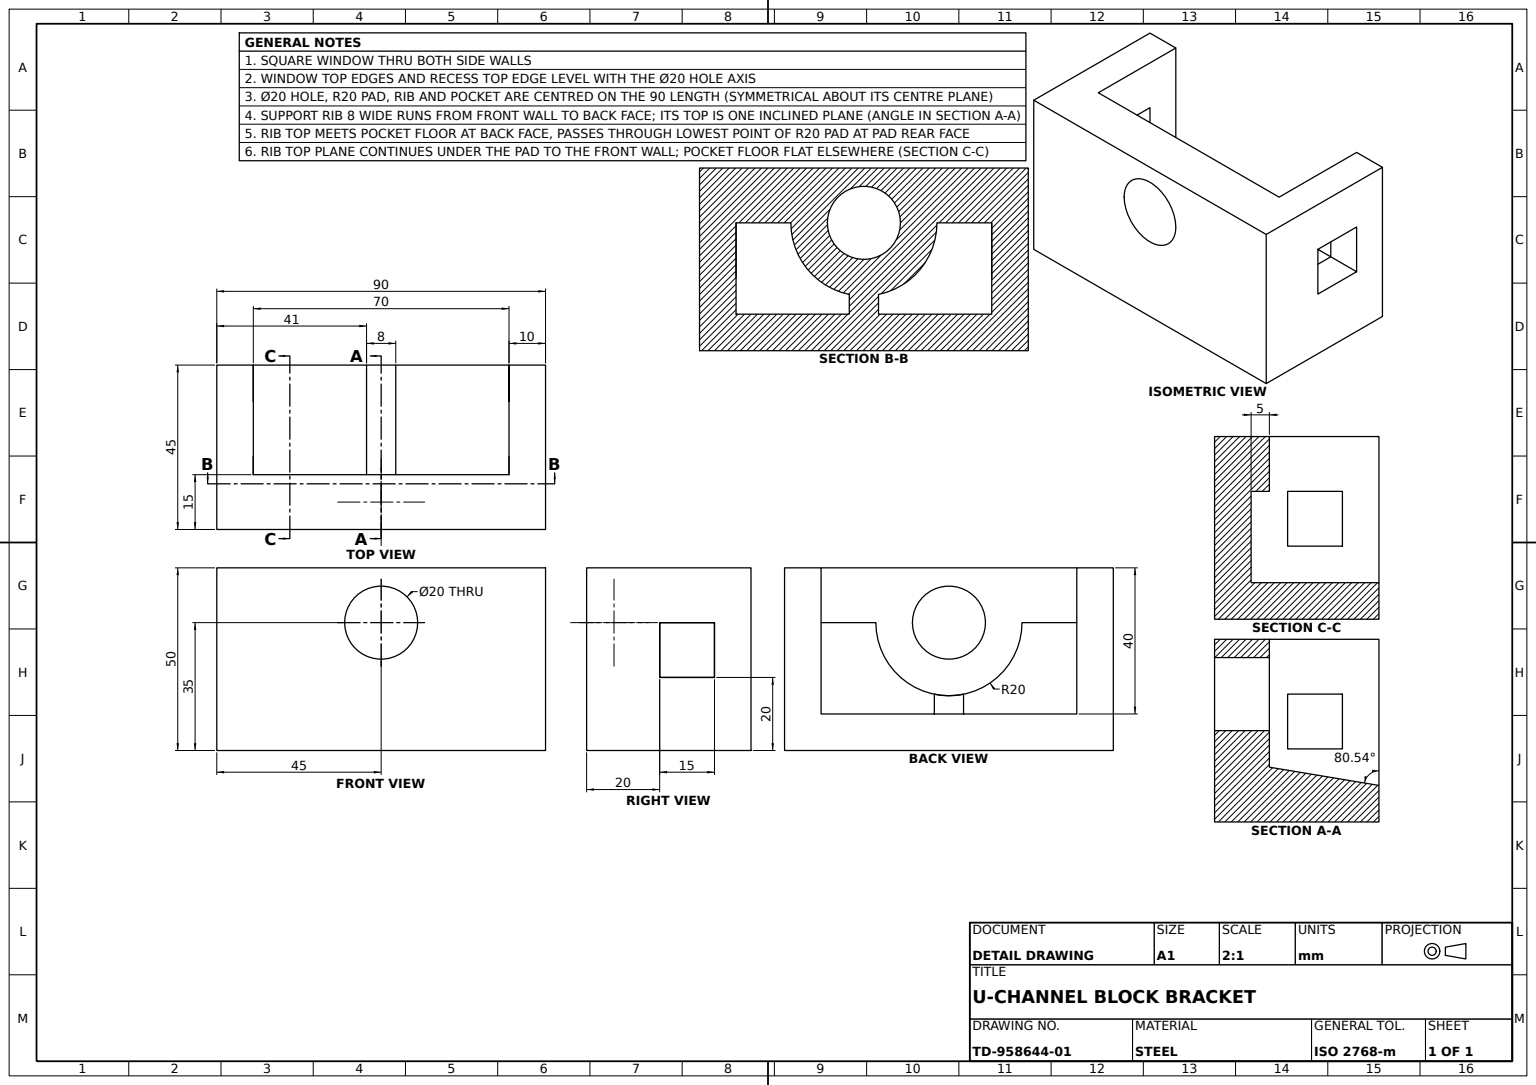
from build123d import *

# Parameters (mm, degrees)
BLOCK_PROFILE_SKETCH_W    = 45
BLOCK_PROFILE_SKETCH_H    = 50
BLOCK_PROFILE_SKETCH_W_2  = 15
BLOCK_PROFILE_SKETCH_H_2  = 15
BLOCK_BODY_90MM_DEPTH     = 45
CENTER_POCKET_SKETCH_W    = 70
CENTER_POCKET_SKETCH_H    = 35
CENTER_POCKET_35X70_DEPTH = 40
POCKET_PAD_SKETCH_R       = 10
POCKET_PAD_5MM_DEPTH      = 5
SIDE_HOLE_REACH           = 64.249
SIDE_HOLE_SKETCH_R        = 10
SUPPORT_RIB_8MM_REACH     = 58.181
SUPPORT_RIB_SKETCH_WALL_W = 144.774837922
SUPPORT_RIB_SKETCH_WALL_H = 8


with BuildPart() as part:
    # Block Profile Sketch → Block Body 90mm (new, symmetric)
    with BuildSketch(Plane(origin=(0, 0, 0), x_dir=(0, 0, -1), z_dir=(1, 0, 0))):
        Rectangle(BLOCK_PROFILE_SKETCH_W, BLOCK_PROFILE_SKETCH_H)
        with Locations((5, 2.5)):
            Rectangle(BLOCK_PROFILE_SKETCH_W_2, BLOCK_PROFILE_SKETCH_H_2, mode=Mode.SUBTRACT)
    extrude(amount=BLOCK_BODY_90MM_DEPTH, both=True)

    # Center Pocket Sketch → Center Pocket 35x70 (cut)
    with BuildSketch(Plane(origin=(0, 25, 0), x_dir=(1, 0, 0), z_dir=(0, 1, 0))):
        with Locations((0, 5)):
            Rectangle(CENTER_POCKET_SKETCH_W, CENTER_POCKET_SKETCH_H)
    extrude(amount=-CENTER_POCKET_35X70_DEPTH, mode=Mode.SUBTRACT)

    # Pocket Pad Sketch → Pocket Pad 5mm (add)
    with BuildSketch(Plane(origin=(0, 0, 12.5), x_dir=(-1, 0, 0), z_dir=(0, 0, -1))):
        with BuildLine():
            Line((20, 10), (35, 10))
            Line((35, 10), (35, 25))
            Line((35, 25), (-35, 25))
            Line((-35, 25), (-35, 10))
            Line((-35, 10), (-20, 10))
            ThreePointArc((-20, 10), (0, -10), (20, 10))
        make_face()
        with Locations((0, 10)):
            Circle(POCKET_PAD_SKETCH_R, mode=Mode.SUBTRACT)
    extrude(amount=POCKET_PAD_5MM_DEPTH)

    # Side Hole Sketch → Side Hole (cut, up to next)
    with BuildSketch(Plane(origin=(0, 0, 12.5), x_dir=(-1, 0, 0), z_dir=(0, 0, -1)), mode=Mode.PRIVATE) as side_hole_sk1:
        with Locations((0, 10)):
            Circle(SIDE_HOLE_SKETCH_R)
    side_hole_tool1 = extrude(side_hole_sk1.sketch, amount=-SIDE_HOLE_REACH, mode=Mode.PRIVATE) & part.part
    add(side_hole_tool1.solids().sort_by_distance((0, 10, 12.5))[0], mode=Mode.SUBTRACT)

    # Support Rib Sketch wall → Support Rib 8mm (add, up to next)
    with BuildSketch(Plane(origin=(0, -12.5, -7.5), x_dir=(0, -0.164398987305, -0.986393923832), z_dir=(0, 0.986393923832, -0.164398987305)), mode=Mode.PRIVATE) as support_rib_8mm_sk1:
        Rectangle(SUPPORT_RIB_SKETCH_WALL_W, SUPPORT_RIB_SKETCH_WALL_H)
    support_rib_8mm_tool1 = extrude(support_rib_8mm_sk1.sketch, amount=-SUPPORT_RIB_8MM_REACH, mode=Mode.PRIVATE) - part.part
    add(support_rib_8mm_tool1.solids().sort_by_distance((0, -12.5, -7.5))[0])


solid = part.part
